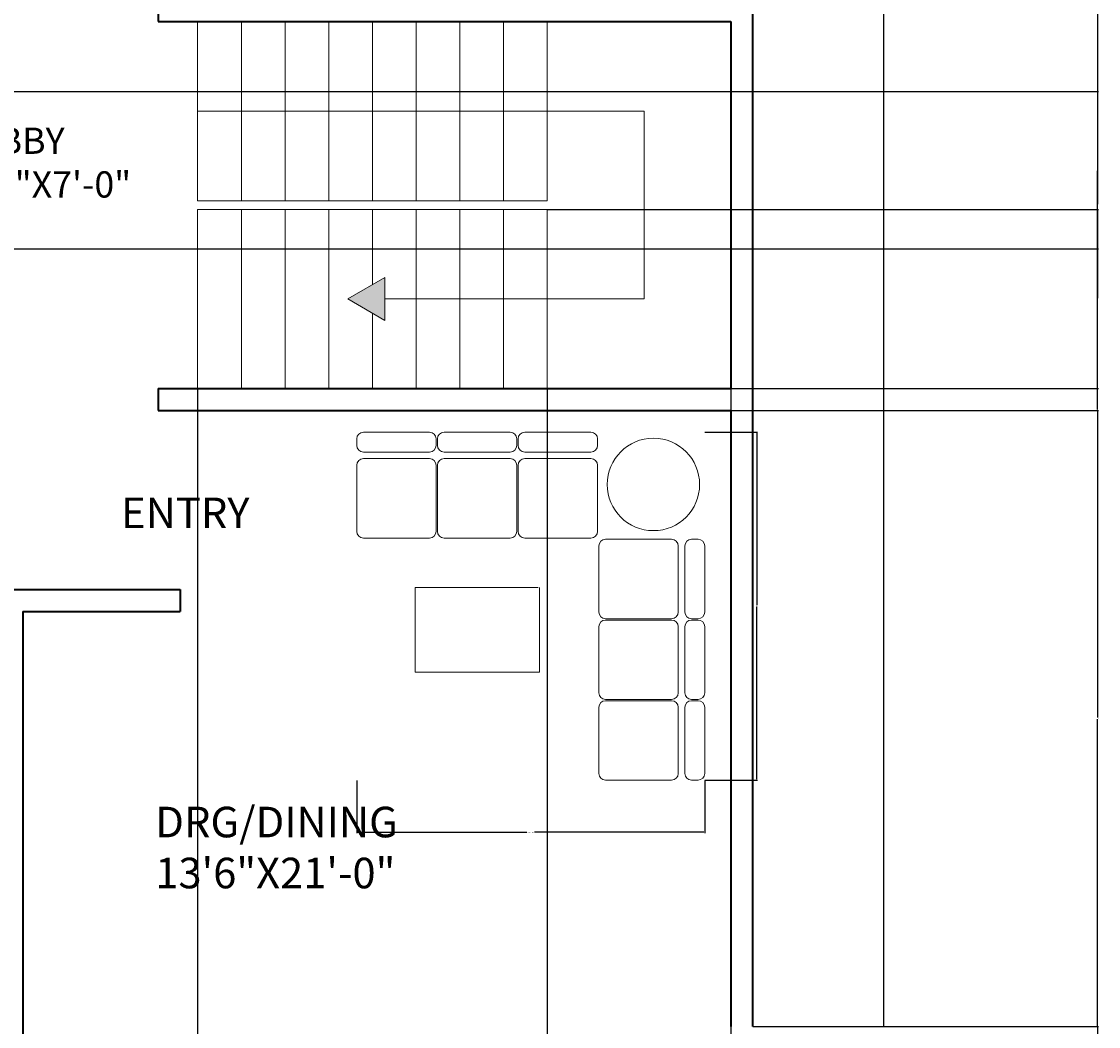
# Model space of a CAD drawing. Units: inches. Extents: x 3731 to 4318, y 1310 to 2388.
# Tile 32 of 57: x 4072 to 4318, y 1708 to 1938. Entities that reach past the tile are written whole.
import ezdxf

# ---------------------------------------------------------------- set-up
doc = ezdxf.new("R2010")
doc.units = ezdxf.units.IN
for name, color, linetype, lineweight in [('A-ANNO-DIMS', 2, 'Continuous', 18), ('A-ANNO-SYMB', 7, 'Continuous', 18), ('A-ANNO-TEXT', 7, 'Continuous', 18), ('A-AREA-IDEN', 7, 'Continuous', 18), ('A-FLOR-STRS', 3, 'Continuous', 18), ('A-FURN', 8, 'Continuous', 13), ('A-WALL', 7, 'Continuous', 35)]:
    doc.layers.add(name, color=color, linetype=linetype, lineweight=lineweight)
doc.styles.get("Standard").update_dxf_attribs({"font": 'arial.ttf'})
doc.dimstyles.get("Standard").update_dxf_attribs({"dimtxt": 0.18, "dimasz": 0.18, "dimexe": 0.18, "dimexo": 0.0625, "dimgap": 0.09, "dimtad": 0, "dimtih": 1, "dimtoh": 1, "dimdec": 4, "dimzin": 0, "dimdsep": 46, "dimtxsty": 'Standard', "dimcen": 0.09, "dimadec": 0, "dimazin": 0, "dimtfac": 1, "dimtdec": 4, "dimtofl": 0, "dimtmove": 0, "dimatfit": 3, "dimfxl": 1, "dimtolj": 1, "dimtzin": 0, "dimarcsym": 0})

# ---------------------------------------------------------------- blocks, each defined once
blk = doc.blocks.new('A$C753D6792')
at = {"linetype": 'ByBlock'}
for p, q in [((50, 2630), (550, 2630)), ((660, 2630), (1160, 2630)), ((1270, 2630), (1770, 2630)), ((0, 2530), (0, 2580)), ((600, 2580), (600, 2530)), ((610, 2530), (610, 2580)), ((1210, 2580), (1210, 2530)), ((1220, 2530), (1220, 2580)), ((1820, 2580), (1820, 2530)), ((550, 2480), (50, 2480)), ((1160, 2480), (660, 2480)), ((1770, 2480), (1270, 2480)), ((0, 1880), (0, 2380)), ((550, 2430), (50, 2430)), ((600, 2380), (600, 1880)), ((610, 1880), (610, 2380)), ((1160, 2430), (660, 2430)), ((1210, 2380), (1210, 1880)), ((1220, 1880), (1220, 2380)), ((1770, 2430), (1270, 2430)), ((1820, 1880), (1820, 2380)), ((50, 1830), (427.2, 1830)), ((386.5, 1830), (550, 1830)), ((660, 1830), (1037.2, 1830)), ((996.5, 1830), (1160, 1830)), ((1270, 1830), (1647.2, 1830)), ((1606.5, 1830), (1770, 1830)), ((1880, 1820), (2380, 1820)), ((2530, 1820), (2580, 1820)), ((1830, 1770), (1830, 1392.8)), ((2430, 1270), (2430, 1770)), ((2480, 1270), (2480, 1770)), ((2630, 1770), (2630, 1270)), ((442.3, 815), (442.3, 1455)), ((442.3, 1455), (1372.3, 1455)), ((1382.3, 1455), (1382.3, 815)), ((1830, 1433.5), (1830, 1270)), ((1830, 1160), (1830, 782.8)), ((2380, 1220), (1880, 1220)), ((1880, 1210), (2380, 1210)), ((2430, 660), (2430, 1160)), ((2480, 660), (2480, 1160)), ((2580, 1220), (2530, 1220)), ((2530, 1210), (2580, 1210)), ((2630, 1160), (2630, 660)), ((1382.3, 815), (442.3, 815)), ((1830, 823.5), (1830, 660)), ((2380, 610), (1880, 610)), ((1880, 600), (2380, 600)), ((2580, 610), (2530, 610)), ((2530, 600), (2580, 600)), ((1830, 550), (1830, 172.8)), ((2430, 50), (2430, 550)), ((2480, 50), (2480, 550)), ((2630, 550), (2630, 50)), ((1830, 213.5), (1830, 50)), ((2380, 0), (1880, 0)), ((2580, 0), (2530, 0))]:
    blk.add_line(p, q, dxfattribs=at)
blk.add_circle((2242.3, 2235), 349.3, dxfattribs=at)
for centre, start, end in [((50, 2580), 90, 180), ((550, 2580), 0, 90), ((550, 2580), 0, 90), ((660, 2580), 90, 180), ((1160, 2580), 0, 90), ((1160, 2580), 0, 90), ((1270, 2580), 90, 180), ((1770, 2580), 0, 90), ((1770, 2580), 0, 90), ((50, 2530), 180, 270), ((550, 2530), 270, 0), ((550, 2530), 270, 0), ((660, 2530), 180, 270), ((1160, 2530), 270, 0), ((1160, 2530), 270, 0), ((1270, 2530), 180, 270), ((1770, 2530), 270, 0), ((1770, 2530), 270, 0), ((50, 2380), 90, 180), ((550, 2380), 0, 90), ((550, 2380), 0, 90), ((660, 2380), 90, 180), ((1160, 2380), 0, 90), ((1160, 2380), 0, 90), ((1270, 2380), 90, 180), ((1770, 2380), 0, 90), ((1770, 2380), 0, 90), ((50, 1880), 180, 270), ((550, 1880), 270, 0), ((660, 1880), 180, 270), ((1160, 1880), 270, 0), ((1270, 1880), 180, 270), ((1770, 1880), 270, 0), ((1880, 1770), 90, 180), ((2380, 1770), 0, 90), ((2530, 1770), 90, 180), ((2580, 1770), 0, 90), ((1880, 1270), 180, 270), ((2380, 1270), 270, 0), ((2380, 1270), 270, 0), ((2530, 1270), 180, 270), ((2530, 1270), 180, 270), ((2580, 1270), 270, 0), ((2580, 1270), 270, 0), ((1880, 1160), 90, 180), ((2380, 1160), 0, 90), ((2530, 1160), 90, 180), ((2580, 1160), 0, 90), ((1880, 660), 180, 270), ((2380, 660), 270, 0), ((2380, 660), 270, 0), ((2530, 660), 180, 270), ((2530, 660), 180, 270), ((2580, 660), 270, 0), ((2580, 660), 270, 0), ((1880, 550), 90, 180), ((2380, 550), 0, 90), ((2530, 550), 90, 180), ((2580, 550), 0, 90), ((1880, 50), 180, 270), ((2380, 50), 270, 0), ((2380, 50), 270, 0), ((2530, 50), 180, 270), ((2530, 50), 180, 270), ((2580, 50), 270, 0), ((2580, 50), 270, 0)]:
    blk.add_arc(centre, 50, start, end, dxfattribs=at)
blk = doc.blocks.new('*D22')
at = {"layer": 'A-ANNO-DIMS', "color": 0, "lineweight": -2, "transparency": 16777216}
for p, q in [((4148.62, 1764.71), (4148.62, 1752.65)), ((4228.25, 1764.71), (4228.25, 1752.65)), ((4148.8, 1752.83), (4187.56, 1752.83)), ((4228.07, 1752.83), (4189.31, 1752.83))]:
    blk.add_line(p, q, dxfattribs=at)
at = {"layer": 'A-ANNO-DIMS', "color": 0, "transparency": 16777216}
for points in [[(4148.8, 1752.86), (4148.8, 1752.8), (4148.62, 1752.83)], [(4228.07, 1752.86), (4228.07, 1752.8), (4228.25, 1752.83)]]:
    blk.add_solid(points, dxfattribs=at)
at = {"layer": 'Defpoints', "color": 0, "transparency": 16777216}
for p in [(4148.62, 1764.77), (4228.25, 1764.77), (4228.25, 1752.83)]:
    blk.add_point(p, dxfattribs=at)
at = {"layer": 'A-ANNO-DIMS', "color": 0, "transparency": 16777216, "insert": (4188.44, 1752.83), "char_height": 0.18, "attachment_point": 5}
blk.add_mtext('\\A1;SOFA SET 80', dxfattribs=at)
blk = doc.blocks.new('*D23')
at = {"layer": 'A-ANNO-DIMS', "color": 0, "lineweight": -2, "transparency": 16777216}
for p, q in [((4228.31, 1844.4), (4240.37, 1844.4)), ((4240.19, 1844.22), (4240.19, 1804.77)), ((4240.19, 1764.95), (4240.19, 1804.4)), ((4228.31, 1764.77), (4240.37, 1764.77))]:
    blk.add_line(p, q, dxfattribs=at)
at = {"layer": 'A-ANNO-DIMS', "color": 0, "transparency": 16777216}
for points in [[(4240.16, 1844.22), (4240.22, 1844.22), (4240.19, 1844.4)], [(4240.16, 1764.95), (4240.22, 1764.95), (4240.19, 1764.77)]]:
    blk.add_solid(points, dxfattribs=at)
at = {"layer": 'Defpoints', "color": 0, "transparency": 16777216}
for p in [(4228.25, 1844.4), (4240.19, 1844.4), (4228.25, 1764.77)]:
    blk.add_point(p, dxfattribs=at)
at = {"layer": 'A-ANNO-DIMS', "color": 0, "transparency": 16777216, "insert": (4240.19, 1804.58), "char_height": 0.18, "attachment_point": 5}
blk.add_mtext('\\A1;80', dxfattribs=at)
blk = doc.blocks.new('*D39')
at = {"layer": 'A-ANNO-DIMS', "color": 0, "lineweight": -2, "transparency": 16777216}
for p, q in [((4234.27, 1943.38), (4318.34, 1943.38)), ((4318.16, 1943.2), (4318.16, 1896.56)), ((4318.16, 1849.56), (4318.16, 1896.2)), ((4234.27, 1849.38), (4318.34, 1849.38))]:
    blk.add_line(p, q, dxfattribs=at)
at = {"layer": 'A-ANNO-DIMS', "color": 0, "transparency": 16777216}
for points in [[(4318.13, 1943.2), (4318.19, 1943.2), (4318.16, 1943.38)], [(4318.13, 1849.56), (4318.19, 1849.56), (4318.16, 1849.38)]]:
    blk.add_solid(points, dxfattribs=at)
at = {"layer": 'Defpoints', "color": 0, "transparency": 16777216}
for p in [(4234.21, 1943.38), (4318.16, 1943.38), (4234.21, 1849.38)]:
    blk.add_point(p, dxfattribs=at)
at = {"layer": 'A-ANNO-DIMS', "color": 0, "transparency": 16777216, "insert": (4318.16, 1896.38), "char_height": 0.18, "attachment_point": 5}
blk.add_mtext('\\A1;94', dxfattribs=at)
blk = doc.blocks.new('*D40')
at = {"layer": 'A-ANNO-DIMS', "color": 0, "lineweight": -2, "transparency": 16777216}
for p, q in [((4234.27, 1849.38), (4318.34, 1849.38)), ((4318.16, 1849.2), (4318.16, 1779.06)), ((4318.16, 1708.56), (4318.16, 1778.7)), ((4239.27, 1708.38), (4318.34, 1708.38))]:
    blk.add_line(p, q, dxfattribs=at)
at = {"layer": 'A-ANNO-DIMS', "color": 0, "transparency": 16777216}
for points in [[(4318.13, 1849.2), (4318.19, 1849.2), (4318.16, 1849.38)], [(4318.13, 1708.56), (4318.19, 1708.56), (4318.16, 1708.38)]]:
    blk.add_solid(points, dxfattribs=at)
at = {"layer": 'Defpoints', "color": 0, "transparency": 16777216}
for p in [(4234.21, 1849.38), (4318.16, 1849.38), (4239.21, 1708.38)]:
    blk.add_point(p, dxfattribs=at)
at = {"layer": 'A-ANNO-DIMS', "color": 0, "transparency": 16777216, "insert": (4318.16, 1778.88), "char_height": 0.18, "attachment_point": 5}
blk.add_mtext('\\A1;141', dxfattribs=at)
blk = doc.blocks.new('*D41')
at = {"layer": 'A-ANNO-DIMS', "color": 0, "lineweight": -2, "transparency": 16777216}
for p, q in [((4269.27, 1708.38), (4318.34, 1708.38)), ((4318.16, 1708.2), (4318.16, 1650.56)), ((4318.16, 1592.56), (4318.16, 1650.2)), ((4269.27, 1592.38), (4318.34, 1592.38))]:
    blk.add_line(p, q, dxfattribs=at)
at = {"layer": 'A-ANNO-DIMS', "color": 0, "transparency": 16777216}
for points in [[(4318.13, 1708.2), (4318.19, 1708.2), (4318.16, 1708.38)], [(4318.13, 1592.56), (4318.19, 1592.56), (4318.16, 1592.38)]]:
    blk.add_solid(points, dxfattribs=at)
at = {"layer": 'Defpoints', "color": 0, "transparency": 16777216}
for p in [(4269.21, 1708.38), (4318.16, 1708.38), (4269.21, 1592.38)]:
    blk.add_point(p, dxfattribs=at)
at = {"layer": 'A-ANNO-DIMS', "color": 0, "transparency": 16777216, "insert": (4318.16, 1650.38), "char_height": 0.18, "attachment_point": 5}
blk.add_mtext('\\A1;116', dxfattribs=at)
blk = doc.blocks.new('*D46')
at = {"layer": 'A-ANNO-DIMS', "color": 0, "lineweight": -2, "transparency": 16777216}
for p, q in [((4112.21, 1854.32), (4112.21, 1310.25)), ((4192.21, 1854.32), (4192.21, 1310.25)), ((4112.39, 1310.43), (4151.99, 1310.43)), ((4192.03, 1310.43), (4152.43, 1310.43))]:
    blk.add_line(p, q, dxfattribs=at)
at = {"layer": 'A-ANNO-DIMS', "color": 0, "transparency": 16777216}
for points in [[(4112.39, 1310.46), (4112.39, 1310.4), (4112.21, 1310.43)], [(4192.03, 1310.46), (4192.03, 1310.4), (4192.21, 1310.43)]]:
    blk.add_solid(points, dxfattribs=at)
at = {"layer": 'Defpoints', "color": 0, "transparency": 16777216}
for p in [(4112.21, 1854.38), (4192.21, 1854.38), (4192.21, 1310.43)]:
    blk.add_point(p, dxfattribs=at)
at = {"layer": 'A-ANNO-DIMS', "color": 0, "transparency": 16777216, "insert": (4152.21, 1310.43), "char_height": 0.18, "attachment_point": 5}
blk.add_mtext('\\A1;80', dxfattribs=at)
blk = doc.blocks.new('*D47')
at = {"layer": 'A-ANNO-DIMS', "color": 0, "lineweight": -2, "transparency": 16777216}
for p, q in [((4192.21, 1854.32), (4192.21, 1310.25)), ((4234.21, 1854.32), (4234.21, 1310.25)), ((4192.39, 1310.43), (4212.99, 1310.43)), ((4234.03, 1310.43), (4213.43, 1310.43))]:
    blk.add_line(p, q, dxfattribs=at)
at = {"layer": 'A-ANNO-DIMS', "color": 0, "transparency": 16777216}
for points in [[(4192.39, 1310.46), (4192.39, 1310.4), (4192.21, 1310.43)], [(4234.03, 1310.46), (4234.03, 1310.4), (4234.21, 1310.43)]]:
    blk.add_solid(points, dxfattribs=at)
at = {"layer": 'Defpoints', "color": 0, "transparency": 16777216}
for p in [(4192.21, 1854.38), (4234.21, 1854.38), (4234.21, 1310.43)]:
    blk.add_point(p, dxfattribs=at)
at = {"layer": 'A-ANNO-DIMS', "color": 0, "transparency": 16777216, "insert": (4213.21, 1310.43), "char_height": 0.18, "attachment_point": 5}
blk.add_mtext('\\A1;42', dxfattribs=at)
blk = doc.blocks.new('*D48')
at = {"layer": 'A-ANNO-DIMS', "color": 0, "lineweight": -2, "transparency": 16777216}
for p, q in [((4192.27, 1895.38), (4318.34, 1895.38)), ((4318.16, 1895.2), (4318.16, 1875.06)), ((4318.16, 1854.56), (4318.16, 1874.7)), ((4192.27, 1854.38), (4318.34, 1854.38))]:
    blk.add_line(p, q, dxfattribs=at)
at = {"layer": 'A-ANNO-DIMS', "color": 0, "transparency": 16777216}
for points in [[(4318.13, 1895.2), (4318.19, 1895.2), (4318.16, 1895.38)], [(4318.13, 1854.56), (4318.19, 1854.56), (4318.16, 1854.38)]]:
    blk.add_solid(points, dxfattribs=at)
at = {"layer": 'Defpoints', "color": 0, "transparency": 16777216}
for p in [(4192.21, 1895.38), (4318.16, 1895.38), (4192.21, 1854.38)]:
    blk.add_point(p, dxfattribs=at)
at = {"layer": 'A-ANNO-DIMS', "color": 0, "transparency": 16777216, "insert": (4318.16, 1874.88), "char_height": 0.18, "attachment_point": 5}
blk.add_mtext('\\A1;41', dxfattribs=at)
blk = doc.blocks.new('*D50')
at = {"layer": 'A-ANNO-DIMS', "color": 0, "lineweight": -2, "transparency": 16777216}
for p, q in [((4029.27, 1922.38), (4318.34, 1922.38)), ((4318.16, 1922.2), (4318.16, 1904.56)), ((4318.16, 1886.56), (4318.16, 1904.2)), ((4029.27, 1886.38), (4318.34, 1886.38))]:
    blk.add_line(p, q, dxfattribs=at)
at = {"layer": 'A-ANNO-DIMS', "color": 0, "transparency": 16777216}
for points in [[(4318.13, 1922.2), (4318.19, 1922.2), (4318.16, 1922.38)], [(4318.13, 1886.56), (4318.19, 1886.56), (4318.16, 1886.38)]]:
    blk.add_solid(points, dxfattribs=at)
at = {"layer": 'Defpoints', "color": 0, "transparency": 16777216}
for p in [(4029.21, 1922.38), (4318.16, 1922.38), (4029.21, 1886.38)]:
    blk.add_point(p, dxfattribs=at)
at = {"layer": 'A-ANNO-DIMS', "color": 0, "transparency": 16777216, "insert": (4318.16, 1904.38), "char_height": 0.18, "attachment_point": 5}
blk.add_mtext('\\A1;36', dxfattribs=at)
blk = doc.blocks.new('*D51')
at = {"layer": 'A-ANNO-DIMS', "color": 0, "lineweight": -2, "transparency": 16777216}
for p, q in [((4239.21, 1708.44), (4239.21, 2387.51)), ((4239.39, 2387.33), (4253.99, 2387.33)), ((4269.03, 2387.33), (4254.43, 2387.33)), ((4269.21, 1708.44), (4269.21, 2387.51))]:
    blk.add_line(p, q, dxfattribs=at)
at = {"layer": 'A-ANNO-DIMS', "color": 0, "transparency": 16777216}
for points in [[(4239.39, 2387.36), (4239.39, 2387.3), (4239.21, 2387.33)], [(4269.03, 2387.36), (4269.03, 2387.3), (4269.21, 2387.33)]]:
    blk.add_solid(points, dxfattribs=at)
at = {"layer": 'Defpoints', "color": 0, "transparency": 16777216}
for p in [(4269.21, 2387.33), (4239.21, 1708.38), (4269.21, 1708.38)]:
    blk.add_point(p, dxfattribs=at)
at = {"layer": 'A-ANNO-DIMS', "color": 0, "transparency": 16777216, "insert": (4254.21, 2387.33), "char_height": 0.18, "attachment_point": 5}
blk.add_mtext('\\A1;30', dxfattribs=at)

msp = doc.modelspace()

# ---------------------------------------------------------------- hatches: boundary and pattern name
at = {"layer": 'A-ANNO-SYMB'}
h = msp.add_hatch(color=256, dxfattribs=at)
h.dxf.hatch_style = 1
h.paths.add_polyline_path([(4155.04, 1879.79), (4146.55, 1874.88), (4155.04, 1869.98)])

# ---------------------------------------------------------------- linework, layer by layer
for p, q in [((4112.21, 1917.88), (4214.42, 1917.88)), ((4214.42, 1917.88), (4214.42, 1874.88)), ((4155.04, 1874.88), (4214.42, 1874.88))]:
    msp.add_line(p, q, dxfattribs=at)
msp.add_lwpolyline([(4146.55, 1874.88), (4155.04, 1869.98), (4155.04, 1879.79)], close=True, dxfattribs=at)
at = {"layer": 'A-FLOR-STRS'}
for p, q in [((4112.21, 1938.38), (4112.21, 1897.38)), ((4122.21, 1938.38), (4122.21, 1897.38)), ((4132.21, 1938.38), (4132.21, 1897.38)), ((4142.21, 1938.38), (4142.21, 1897.38)), ((4152.21, 1938.38), (4152.21, 1897.38)), ((4162.21, 1938.38), (4162.21, 1897.38)), ((4172.21, 1938.38), (4172.21, 1897.38)), ((4182.21, 1938.38), (4182.21, 1897.38)), ((4192.21, 1938.38), (4192.21, 1897.38)), ((4112.21, 1897.38), (4192.21, 1897.38)), ((4112.21, 1895.38), (4192.21, 1895.38)), ((4112.21, 1895.38), (4112.21, 1854.38)), ((4122.21, 1895.38), (4122.21, 1854.38)), ((4132.21, 1895.38), (4132.21, 1854.38)), ((4142.21, 1895.38), (4142.21, 1854.38)), ((4152.21, 1895.38), (4152.21, 1878.15)), ((4162.21, 1895.38), (4162.21, 1854.38)), ((4172.21, 1895.38), (4172.21, 1854.38)), ((4182.21, 1895.38), (4182.21, 1854.38)), ((4192.21, 1895.38), (4192.21, 1854.38)), ((4152.21, 1871.61), (4152.21, 1854.38))]:
    msp.add_line(p, q, dxfattribs=at)
at = {"layer": 'A-WALL'}
for p, q in [((4239.21, 2338.38), (4239.21, 1708.38)), ((4103.21, 2074.38), (4103.21, 1938.38)), ((4103.21, 1938.38), (4234.21, 1938.38)), ((4234.21, 1938.38), (4234.21, 1854.38)), ((4103.21, 1854.38), (4234.21, 1854.38)), ((4103.21, 1854.38), (4103.21, 1849.38)), ((4103.21, 1849.38), (4234.21, 1849.38)), ((4187.21, 1849.45), (4187.21, 1849.38)), ((4192.21, 1849.45), (4192.21, 1849.38)), ((4234.21, 1849.38), (4234.21, 1708.38)), ((4033.21, 1808.38), (4108.21, 1808.38)), ((4108.21, 1808.38), (4108.21, 1803.38)), ((4072.21, 1803.38), (4072.21, 1484.38)), ((4072.21, 1803.38), (4108.21, 1803.38))]:
    msp.add_line(p, q, dxfattribs=at)

# ---------------------------------------------------------------- block references
at = {"layer": 'A-FURN', "xscale": 0.0302759400746394, "yscale": 0.0302759400746394, "zscale": 0.0302759400746394}
msp.add_blockref('A$C753D6792', (4148.62, 1764.77), dxfattribs=at)

# ---------------------------------------------------------------- texts
at = {"layer": 'A-ANNO-TEXT', "insert": (4094.69, 1829.43), "char_height": 7, "attachment_point": 1}
msp.add_mtext_dynamic_manual_height_columns('ENTRY', width=10.4564, gutter_width=12.5, heights=[0], dxfattribs=at)
at = {"layer": 'A-AREA-IDEN', "attachment_point": 1}
for s, insert, char_height in [('LOBBY\\P7\'-6"X7\'-0"', (4056.14, 1914.1), 6), ('DRG/DINING\\P13\'6"X21\'-0"', (4102.51, 1758.67), 7)]:
    msp.add_mtext_dynamic_manual_height_columns(s, width=47.0437, gutter_width=12.5, heights=[0], dxfattribs=dict(at, insert=insert, char_height=char_height))

# ---------------------------------------------------------------- dimensions: what is measured, and where the dimension line sits
at = {"layer": 'A-ANNO-DIMS'}
for base, p1, p2, picture, middle in [((4269.21, 2387.33), (4239.21, 1708.38), (4269.21, 1708.38), '*D51', (4254.21, 2387.33)), ((4192.21, 1310.43), (4112.21, 1854.38), (4192.21, 1854.38), '*D46', (4152.21, 1310.43)), ((4234.21, 1310.43), (4192.21, 1854.38), (4234.21, 1854.38), '*D47', (4213.21, 1310.43))]:
    dim = msp.add_linear_dim(base=base, p1=p1, p2=p2, dimstyle='Standard', override={"dimdec": 0, "dimlfac": 1, "dimrnd": 0, "dimzin": 0, "dimdsep": 46, "dimlunit": 2}, dxfattribs=at)
    dim.commit()
    dim.dimension.update_dxf_attribs({"geometry": picture, "text_midpoint": middle})
for base, p1, p2, picture, middle in [((4318.16, 1943.38), (4234.21, 1849.38), (4234.21, 1943.38), '*D39', (4318.16, 1896.38)), ((4318.16, 1922.38), (4029.21, 1886.38), (4029.21, 1922.38), '*D50', (4318.16, 1904.38)), ((4318.16, 1895.38), (4192.21, 1854.38), (4192.21, 1895.38), '*D48', (4318.16, 1874.88)), ((4318.16, 1849.38), (4239.21, 1708.38), (4234.21, 1849.38), '*D40', (4318.16, 1778.88)), ((4240.19, 1844.4), (4228.25, 1764.77), (4228.25, 1844.4), '*D23', (4240.19, 1804.58)), ((4318.16, 1708.38), (4269.21, 1592.38), (4269.21, 1708.38), '*D41', (4318.16, 1650.38))]:
    dim = msp.add_linear_dim(base=base, p1=p1, p2=p2, angle=90, dimstyle='Standard', override={"dimdec": 0, "dimlfac": 1, "dimrnd": 0, "dimzin": 0, "dimdsep": 46, "dimlunit": 2}, dxfattribs=at)
    dim.commit()
    dim.dimension.update_dxf_attribs({"geometry": picture, "text_midpoint": middle})
dim = msp.add_linear_dim(base=(4228.25, 1752.83), p1=(4148.62, 1764.77), p2=(4228.25, 1764.77), text='SOFA SET <>', dimstyle='Standard', override={"dimdec": 0, "dimlfac": 1, "dimrnd": 0, "dimzin": 0, "dimdsep": 46, "dimlunit": 2}, dxfattribs=at)
dim.commit()
dim.dimension.update_dxf_attribs({"geometry": '*D22', "text_midpoint": (4188.44, 1752.83)})

doc.saveas('drawing.dxf')
